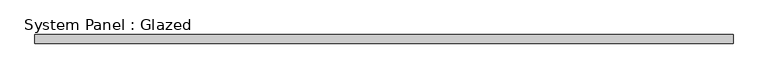
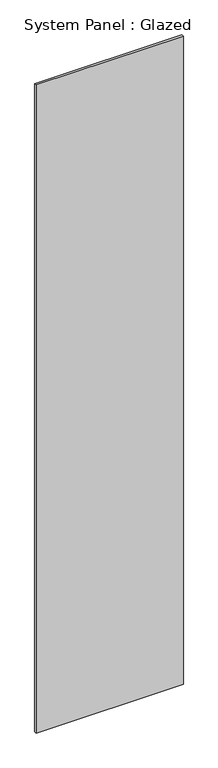
"""IFC4 building model written with IfcOpenShell, lengths in millimetres: plate geometry, System Panel : Glazed."""

from ifc_helpers import new_model, si_unit, origin, origin_with_axes, place, context, project, spatial, polyline, outline, extrude, source, transform, mapped, element, save


def system_panel_glazed_2f845612(model_context):
    return source(origin(), model_context, "Body", "SweptSolid", [
        extrude(outline(polyline([(984.5872482, 19.05), (-984.5872482, 19.05), (-984.5872482, 44.45), (984.5872482, 44.45), (984.5872482, 19.05)])), origin_with_axes(), (0.0, 0.0, 1.0), 9144.0),
    ])


if __name__ == "__main__":
    model = new_model("IFC4")
    model_context = context("Model", 3, world=origin())
    ifc_project = project(units=[si_unit("LENGTHUNIT", "METRE", prefix="MILLI")], contexts=[model_context])
    site = spatial("IfcSite", under=ifc_project)
    building = spatial("IfcBuilding", under=site)
    placement = place(None, origin())
    system_panel_glazed_shape = system_panel_glazed_2f845612(model_context)
    element("IfcPlate", 1, ObjectType="System Panel : Glazed", at=placement, inside=building, context=model_context, shape_type="MappedRepresentation", body=[
        mapped(system_panel_glazed_shape, transform((0.0, 0.0, 0.0), x_axis=(1.0, 0.0, 0.0), y_axis=(0.0, 1.0, 0.0), z_axis=(0.0, 0.0, 1.0))),
    ])
    save(model, "model.ifc")

# Revit data of these elements
# Type "System Panel : Glazed"
#   Construction Type Id = "GSP4R"
#   Analytic Construction = "1/8 in Pilkington single glazing"
#   Visual Light Transmittance = 0.9
#   Solar Heat Gain Coefficient = 0.86
#   Heat Transfer Coefficient (U) = 1.18115 BTU/(h·ft²·°F)
#   Define Thermal Properties by = 1
# Element 1 (IfcPlate, "System Panel : Glazed")
#   Materials on its faces: "Glass"
# Materials
#   "Glass": class "Glass", colour RGB 0 128 192, transparency 0.75, Description = "Soda Lime Glass", Cost = 0
